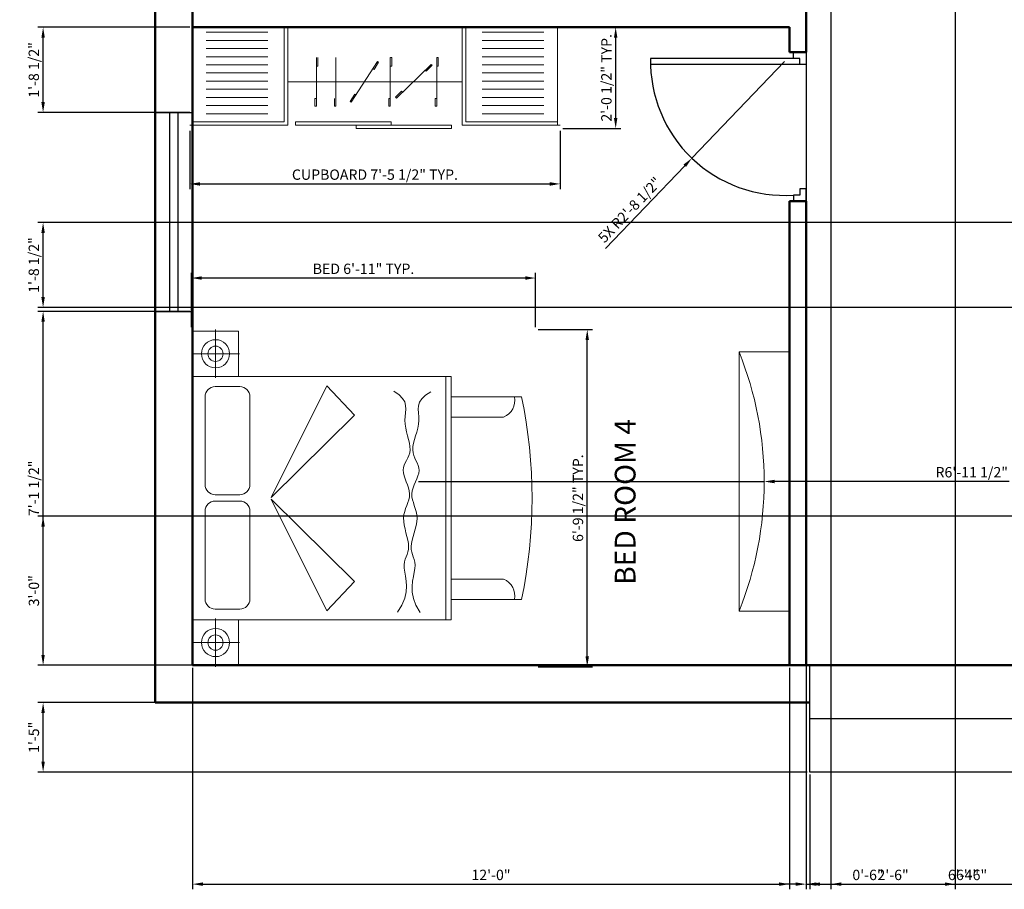
# Model space of a CAD drawing. Units: inches. Extents: x 1905 to 2315, y 3232 to 3824.
# Tile 1 of 8: x 1905 to 2143, y 3232 to 3442. Entities that reach past the tile are written whole.
import ezdxf

# ---------------------------------------------------------------- set-up
doc = ezdxf.new("R2010")
doc.units = ezdxf.units.IN
for name, color, linetype, lineweight in [('A-ANNO-DIMS', 2, 'Continuous', 18), ('A-AREA-IDEN', 7, 'Continuous', 25), ('A-FLOR-CABT', 8, 'Continuous', 18), ('A-FLOR-STRS', 7, 'Continuous', 25), ('A-FURN', 8, 'Continuous', 18), ('door', 1, 'Continuous', 25), ('TV', 221, 'Continuous', 18), ('wall', 2, 'Continuous', 50), ('WINDOW', 60, 'Continuous', 25)]:
    doc.layers.add(name, color=color, linetype=linetype, lineweight=lineweight)
doc.styles.get("Standard").update_dxf_attribs({"font": 'arial.ttf'})
doc.dimstyles.new('ISO-25', dxfattribs={"dimtxt": 2.5, "dimasz": 2.5, "dimexe": 1.25, "dimexo": 0.625, "dimtad": 1, "dimdec": 1, "dimlunit": 3, "dimtxsty": 'Standard', "dimcen": 2.5, "dimadec": 0, "dimazin": 0, "dimtfac": 1, "dimtdec": 1, "dimtmove": 0, "dimatfit": 3, "dimfxl": 1, "dimarcsym": 0})

# ---------------------------------------------------------------- blocks, each defined once
blk = doc.blocks.new('A$C4F543DC7')
for p, q in [((0.0134, 3.35, -0.1688), (3.3134, 3.35, -0.1688)), ((0.4634, 3.35, -0.1688), (0.0134, 3.35, -0.1688)), ((0.0134, 2.896, -0.1688), (0.0134, 3.35, -0.1688)), ((0.0134, 3.35, -0.1688), (0.0134, 2.896, -0.1688)), ((0.2381, 3.1233, -0.4388), (0.2381, 3.3614, -0.4388)), ((0.4634, 3.35, -0.1688), (0.4634, 0.8, -0.1688)), ((2.8634, 3.35, -0.1688), (0.4634, 3.35, -0.1688)), ((0.4634, 2.896, -0.1688), (0.4634, 3.35, -0.1688)), ((2.8634, 0.8, -0.1688), (2.8634, 3.35, -0.1688)), ((2.8634, 3.35, -0.1688), (3.3134, 3.35, -0.1688)), ((2.8634, 2.896, -0.1688), (2.8634, 3.35, -0.1688)), ((3.0888, 3.1233, -0.4388), (3.0888, 3.3614, -0.4388)), ((3.3134, 3.35, -0.1688), (3.3134, 2.896, -0.1688)), ((3.3134, 3.35, -0.1688), (3.3134, 2.896, -0.1688)), ((1.5354, 3.226, -0.1688), (0.6684, 3.226, -0.1688)), ((2.6644, 3.226, -0.1688), (1.7974, 3.226, -0.1688)), ((0.2381, 3.1233, -0.4388), (0, 3.1233, -0.4388)), ((0.2381, 3.1233, -0.4388), (0.4762, 3.1233, -0.4388)), ((0.2381, 3.1233, -0.4388), (0.2381, 2.8852, -0.4388)), ((0.5684, 3.126, -0.1688), (0.5684, 2.884, -0.1688)), ((1.6354, 2.884, -0.1688), (1.6354, 3.126, -0.1688)), ((1.6974, 3.126, -0.1688), (1.6974, 2.884, -0.1688)), ((2.7644, 2.884, -0.1688), (2.7644, 3.126, -0.1688)), ((3.0888, 3.1233, -0.4388), (2.8507, 3.1233, -0.4388)), ((3.0888, 3.1233, -0.4388), (3.0888, 2.8852, -0.4388)), ((3.0888, 3.1233, -0.4388), (3.3269, 3.1233, -0.4388)), ((0.4634, 2.896, -0.1688), (0.0134, 2.896, -0.1688)), ((0.0134, 2.896, -0.1688), (0.4634, 2.896, -0.1688)), ((0.4634, 0.8, -0.1688), (0.4634, 2.896, -0.1688)), ((2.8634, 2.896, -0.1688), (2.8634, 0.8, -0.1688)), ((3.3134, 2.896, -0.1688), (2.8634, 2.896, -0.1688)), ((3.3134, 2.896, -0.1688), (2.8634, 2.896, -0.1688)), ((0.6684, 2.784, -0.1688), (1.5354, 2.784, -0.1688)), ((1.7974, 2.784, -0.1688), (2.6644, 2.784, -0.1688)), ((1.6534, 2.573, -0.1688), (0.5504, 2.025, -0.1688)), ((0.8414, 1.752, -0.1688), (1.6534, 2.573, -0.1688)), ((2.4814, 1.752, -0.1688), (1.6694, 2.573, -0.1688)), ((1.6694, 2.573, -0.1688), (2.7724, 2.025, -0.1688)), ((0.5504, 2.025, -0.1688), (0.8414, 1.752, -0.1688)), ((2.7724, 2.025, -0.1688), (2.4814, 1.752, -0.1688)), ((2.683, 1.312, -0.1688), (2.7182, 1.3641, -0.1688)), ((0.5369, 1.3267, -0.1688), (0.6088, 1.2835, -0.1688)), ((0.6088, 1.2835, -0.1688), (0.6756, 1.2566, -0.1688)), ((1.3963, 1.2612, -0.1688), (1.4328, 1.2664, -0.1688)), ((1.4328, 1.2664, -0.1688), (1.4679, 1.2677, -0.1688)), ((1.4679, 1.2677, -0.1688), (1.501, 1.2643, -0.1688)), ((1.501, 1.2643, -0.1688), (1.5324, 1.257, -0.1688)), ((1.8557, 1.2531, -0.1688), (1.8849, 1.263, -0.1688)), ((1.8849, 1.263, -0.1688), (1.913, 1.2698, -0.1688)), ((1.913, 1.2698, -0.1688), (1.9397, 1.2722, -0.1688)), ((1.9397, 1.2722, -0.1688), (1.9649, 1.2692, -0.1688)), ((1.9649, 1.2692, -0.1688), (1.989, 1.2617, -0.1688)), ((2.6129, 1.257, -0.1688), (2.6479, 1.2774, -0.1688)), ((2.6479, 1.2774, -0.1688), (2.683, 1.312, -0.1688)), ((0.6067, 1.1458, -0.1688), (0.6743, 1.1706, -0.1688)), ((0.6743, 1.1706, -0.1688), (0.7364, 1.1825, -0.1688)), ((0.6756, 1.2566, -0.1688), (0.7373, 1.2428, -0.1688)), ((0.7364, 1.1825, -0.1688), (0.7931, 1.1846, -0.1688)), ((0.7373, 1.2428, -0.1688), (0.794, 1.239, -0.1688)), ((0.7931, 1.1846, -0.1688), (0.8447, 1.1799, -0.1688)), ((0.794, 1.239, -0.1688), (0.8457, 1.242, -0.1688)), ((0.8447, 1.1799, -0.1688), (0.8913, 1.1716, -0.1688)), ((0.8457, 1.242, -0.1688), (0.8925, 1.2489, -0.1688)), ((0.8913, 1.1716, -0.1688), (0.9331, 1.1628, -0.1688)), ((0.8925, 1.2489, -0.1688), (0.9345, 1.2564, -0.1688)), ((0.9345, 1.2564, -0.1688), (0.9718, 1.2615, -0.1688)), ((0.9718, 1.2615, -0.1688), (1.0044, 1.2617, -0.1688)), ((1.0044, 1.2617, -0.1688), (1.0334, 1.2578, -0.1688)), ((1.0334, 1.2578, -0.1688), (1.0597, 1.2509, -0.1688)), ((1.0583, 1.1642, -0.1688), (1.0831, 1.172, -0.1688)), ((1.0597, 1.2509, -0.1688), (1.0842, 1.2424, -0.1688)), ((1.0831, 1.172, -0.1688), (1.1072, 1.18, -0.1688)), ((1.0842, 1.2424, -0.1688), (1.1081, 1.2336, -0.1688)), ((1.1072, 1.18, -0.1688), (1.1316, 1.1872, -0.1688)), ((1.1081, 1.2336, -0.1688), (1.1322, 1.2257, -0.1688)), ((1.1316, 1.1872, -0.1688), (1.1573, 1.192, -0.1688)), ((1.1322, 1.2257, -0.1688), (1.1577, 1.2201, -0.1688)), ((1.1573, 1.192, -0.1688), (1.1851, 1.1932, -0.1688)), ((1.1577, 1.2201, -0.1688), (1.1855, 1.218, -0.1688)), ((1.1851, 1.1932, -0.1688), (1.2158, 1.1898, -0.1688)), ((1.1855, 1.218, -0.1688), (1.2163, 1.2204, -0.1688)), ((1.2158, 1.1898, -0.1688), (1.2491, 1.1828, -0.1688)), ((1.2163, 1.2204, -0.1688), (1.2498, 1.2264, -0.1688)), ((1.2491, 1.1828, -0.1688), (1.2842, 1.1734, -0.1688)), ((1.2498, 1.2264, -0.1688), (1.2852, 1.2347, -0.1688)), ((1.2842, 1.1734, -0.1688), (1.3206, 1.1629, -0.1688)), ((1.2852, 1.2347, -0.1688), (1.3218, 1.2441, -0.1688)), ((1.3218, 1.2441, -0.1688), (1.3591, 1.2533, -0.1688)), ((1.3591, 1.2533, -0.1688), (1.3963, 1.2612, -0.1688)), ((1.5324, 1.257, -0.1688), (1.5624, 1.2473, -0.1688)), ((1.5624, 1.2473, -0.1688), (1.5915, 1.2365, -0.1688)), ((1.5903, 1.1619, -0.1688), (1.6191, 1.1716, -0.1688)), ((1.5915, 1.2365, -0.1688), (1.6199, 1.2259, -0.1688)), ((1.6191, 1.1716, -0.1688), (1.6475, 1.1797, -0.1688)), ((1.6199, 1.2259, -0.1688), (1.6481, 1.2169, -0.1688)), ((1.6475, 1.1797, -0.1688), (1.676, 1.1849, -0.1688)), ((1.6481, 1.2169, -0.1688), (1.6765, 1.2108, -0.1688)), ((1.676, 1.1849, -0.1688), (1.7049, 1.1858, -0.1688)), ((1.6765, 1.2108, -0.1688), (1.7053, 1.209, -0.1688)), ((1.7049, 1.1858, -0.1688), (1.7344, 1.1816, -0.1688)), ((1.7053, 1.209, -0.1688), (1.7349, 1.2124, -0.1688)), ((1.7344, 1.1816, -0.1688), (1.7643, 1.1731, -0.1688)), ((1.7349, 1.2124, -0.1688), (1.7651, 1.2199, -0.1688)), ((1.7643, 1.1731, -0.1688), (1.7944, 1.1619, -0.1688)), ((1.7651, 1.2199, -0.1688), (1.7955, 1.2301, -0.1688)), ((1.7955, 1.2301, -0.1688), (1.8258, 1.2417, -0.1688)), ((1.8258, 1.2417, -0.1688), (1.8557, 1.2531, -0.1688)), ((1.989, 1.2617, -0.1688), (2.0124, 1.2512, -0.1688)), ((2.0124, 1.2512, -0.1688), (2.0359, 1.2391, -0.1688)), ((2.0359, 1.2391, -0.1688), (2.0599, 1.2269, -0.1688)), ((2.0588, 1.1568, -0.1688), (2.0842, 1.167, -0.1688)), ((2.0599, 1.2269, -0.1688), (2.0849, 1.216, -0.1688)), ((2.0842, 1.167, -0.1688), (2.1112, 1.1743, -0.1688)), ((2.0849, 1.216, -0.1688), (2.1117, 1.2077, -0.1688)), ((2.1112, 1.1743, -0.1688), (2.1403, 1.1775, -0.1688)), ((2.1117, 1.2077, -0.1688), (2.1407, 1.2037, -0.1688)), ((2.1403, 1.1775, -0.1688), (2.1718, 1.1755, -0.1688)), ((2.1407, 1.2037, -0.1688), (2.1723, 1.2047, -0.1688)), ((2.1718, 1.1755, -0.1688), (2.2056, 1.1691, -0.1688)), ((2.1723, 1.2047, -0.1688), (2.2062, 1.21, -0.1688)), ((2.2056, 1.1691, -0.1688), (2.2411, 1.1598, -0.1688)), ((2.2062, 1.21, -0.1688), (2.242, 1.2182, -0.1688)), ((2.242, 1.2182, -0.1688), (2.2791, 1.2279, -0.1688)), ((2.2791, 1.2279, -0.1688), (2.3173, 1.2378, -0.1688)), ((2.3173, 1.2378, -0.1688), (2.3558, 1.2465, -0.1688)), ((2.3558, 1.2465, -0.1688), (2.3944, 1.2527, -0.1688)), ((2.3944, 1.2527, -0.1688), (2.4325, 1.255, -0.1688)), ((2.4325, 1.255, -0.1688), (2.4698, 1.2529, -0.1688)), ((2.4698, 1.2529, -0.1688), (2.5064, 1.2488, -0.1688)), ((2.5064, 1.2488, -0.1688), (2.5423, 1.2459, -0.1688)), ((2.5423, 1.2459, -0.1688), (2.5777, 1.2476, -0.1688)), ((2.5777, 1.2476, -0.1688), (2.6129, 1.257, -0.1688)), ((0.5334, 1.105, -0.1688), (0.6067, 1.1458, -0.1688)), ((0.9331, 1.1628, -0.1688), (0.9701, 1.1565, -0.1688)), ((0.9701, 1.1565, -0.1688), (1.0027, 1.1552, -0.1688)), ((1.0027, 1.1552, -0.1688), (1.0318, 1.1582, -0.1688)), ((1.0318, 1.1582, -0.1688), (1.0583, 1.1642, -0.1688)), ((1.3206, 1.1629, -0.1688), (1.3575, 1.1524, -0.1688)), ((1.3575, 1.1524, -0.1688), (1.3945, 1.1434, -0.1688)), ((1.3945, 1.1434, -0.1688), (1.4308, 1.1371, -0.1688)), ((1.4308, 1.1371, -0.1688), (1.4658, 1.1347, -0.1688)), ((1.4658, 1.1347, -0.1688), (1.499, 1.137, -0.1688)), ((1.499, 1.137, -0.1688), (1.5306, 1.1433, -0.1688)), ((1.5306, 1.1433, -0.1688), (1.5609, 1.152, -0.1688)), ((1.5609, 1.152, -0.1688), (1.5903, 1.1619, -0.1688)), ((1.7944, 1.1619, -0.1688), (1.8244, 1.1494, -0.1688)), ((1.8244, 1.1494, -0.1688), (1.8539, 1.137, -0.1688)), ((1.8539, 1.137, -0.1688), (1.8827, 1.1263, -0.1688)), ((1.8827, 1.1263, -0.1688), (1.9106, 1.1186, -0.1688)), ((1.9106, 1.1186, -0.1688), (1.9373, 1.1153, -0.1688)), ((1.9373, 1.1153, -0.1688), (1.9625, 1.1176, -0.1688)), ((1.9625, 1.1176, -0.1688), (1.9868, 1.1243, -0.1688)), ((1.9868, 1.1243, -0.1688), (2.0106, 1.134, -0.1688)), ((2.0106, 1.134, -0.1688), (2.0344, 1.1454, -0.1688)), ((2.0344, 1.1454, -0.1688), (2.0588, 1.1568, -0.1688)), ((2.2411, 1.1598, -0.1688), (2.2779, 1.1489, -0.1688)), ((2.2779, 1.1489, -0.1688), (2.3157, 1.1379, -0.1688)), ((2.3157, 1.1379, -0.1688), (2.354, 1.1279, -0.1688)), ((2.354, 1.1279, -0.1688), (2.3923, 1.1205, -0.1688)), ((2.3923, 1.1205, -0.1688), (2.4304, 1.117, -0.1688)), ((2.4304, 1.117, -0.1688), (2.4677, 1.118, -0.1688)), ((2.4677, 1.118, -0.1688), (2.5043, 1.1209, -0.1688)), ((2.5043, 1.1209, -0.1688), (2.5403, 1.1226, -0.1688)), ((2.5403, 1.1226, -0.1688), (2.5757, 1.1199, -0.1688)), ((2.5757, 1.1199, -0.1688), (2.6106, 1.1094, -0.1688)), ((2.6106, 1.1094, -0.1688), (2.645, 1.0879, -0.1688)), ((2.645, 1.0879, -0.1688), (2.6789, 1.0522, -0.1688)), ((2.6789, 1.0522, -0.1688), (2.7124, 0.999, -0.1688)), ((0.4634, 0.85, -0.1688), (2.8634, 0.85, -0.1688)), ((0.4634, 0.8, -0.1688), (2.8634, 0.8, -0.1688)), ((0.6634, 0.8, -0.1688), (0.4634, 0.8, -0.1688)), ((0.6634, 0.8, -0.1688), (2.6634, 0.8, -0.1688)), ((0.6634, 0.104, -0.1688), (0.6634, 0.8, -0.1688)), ((0.6634, 0.104, -0.1688), (0.6634, 0.8, -0.1688)), ((0.8634, 0.281, -0.1688), (0.8634, 0.8, -0.1688)), ((2.4634, 0.8, -0.1688), (2.4634, 0.281, -0.1688)), ((2.8634, 0.8, -0.1688), (2.6634, 0.8, -0.1688)), ((2.6634, 0.8, -0.1688), (2.6634, 0.104, -0.1688)), ((2.6634, 0.8, -0.1688), (2.6634, 0.104, -0.1688))]:
    blk.add_line(p, q)
for centre, radius in [((0.2381, 3.1233, -0.4388), 0.139), ((3.0888, 3.1233, -0.4388), 0.139), ((0.2381, 3.1233, -0.4388), 0.075), ((3.0888, 3.1233, -0.4388), 0.075)]:
    blk.add_circle(centre, radius)
for centre, radius, start, end in [((0.6684, 3.126, -0.1688), 0.1, 90, 180), ((1.5354, 3.126, -0.1688), 0.1, 0, 90), ((1.7974, 3.126, -0.1688), 0.1, 90, 180), ((2.6644, 3.126, -0.1688), 0.1, 0, 90), ((0.6684, 2.884, -0.1688), 0.1, 180, 270), ((1.5354, 2.884, -0.1688), 0.1, 270, 0), ((1.7974, 2.884, -0.1688), 0.1, 180, 270), ((2.6644, 2.884, -0.1688), 0.1, 270, 0), ((0.6994, 0.3472, -0.1688), 0.1769, 258.2616, 338.03196), ((2.6275, 0.3472, -0.1688), 0.1769, 201.96804, 281.7384), ((1.6634, 4.8597, -0.1688), 4.8597, 258.12517, 281.87483), ((1.6634, 4.8597, -0.1688), 4.8597, 258.12517, 281.87483)]:
    blk.add_arc(centre, radius, start, end)
blk = doc.blocks.new('CUPBOARD-DOUBLE-BAY')
at = {"ltscale": 0.05}
for p, q in [((88.68, 24.41), (0.66, 24.41)), ((0.66, 0.79), (0.66, 24.41)), ((88.68, 0.79), (88.68, 24.41)), ((48.39, 17.11), (48.73, 17.11)), ((59.57, 17.11), (59.9, 17.11)), ((30.53, 15.05), (30.86, 15.05)), ((44.17, 14.43), (44.45, 14.25)), ((45.28, 16.16), (45.56, 15.98)), ((48.39, 15.05), (48.73, 15.05)), ((58.24, 15.47), (58.47, 15.23)), ((59.57, 15.05), (59.9, 15.05)), ((56.76, 14.03), (56.99, 13.79)), ((30.53, 7.22), (30.19, 7.22)), ((40.06, 8.06), (39.78, 8.24)), ((48.35, 7.22), (48.02, 7.22)), ((49.85, 7.29), (49.61, 7.53)), ((51.32, 8.73), (51.09, 8.97)), ((59.57, 7.22), (59.23, 7.22)), ((30.53, 5.41), (30.19, 5.41)), ((35.23, 5.41), (34.9, 5.41)), ((38.95, 6.33), (38.67, 6.51)), ((48.35, 5.41), (48.02, 5.41)), ((59.57, 5.41), (59.23, 5.41))]:
    blk.add_line(p, q, dxfattribs=at)
for p, q in [((22.77, 1.58), (22.77, 24.41)), ((23.62, 0.79), (23.62, 24.41)), ((65.72, 0.79), (65.72, 24.41)), ((66.57, 1.58), (66.57, 24.41)), ((18.83, 23.23), (3.94, 23.23)), ((70.51, 23.23), (85.4, 23.23)), ((18.83, 21.26), (3.94, 21.26)), ((18.83, 19.29), (3.94, 19.29)), ((70.51, 21.26), (85.4, 21.26)), ((70.51, 19.29), (85.4, 19.29)), ((18.83, 17.32), (3.94, 17.32)), ((30.53, 5.41), (30.53, 17.11)), ((30.86, 15.05), (30.86, 17.11)), ((35.23, 5.41), (35.23, 17.11)), ((48.35, 5.41), (48.35, 17.11)), ((48.73, 15.05), (48.73, 17.11)), ((59.57, 5.41), (59.57, 17.11)), ((59.9, 15.05), (59.9, 17.11)), ((70.51, 17.32), (85.4, 17.32)), ((18.83, 15.35), (3.94, 15.35)), ((38.95, 6.33), (45.28, 16.16)), ((44.45, 14.25), (45.56, 15.98)), ((49.85, 7.29), (58.22, 15.46)), ((56.99, 13.79), (58.47, 15.23)), ((70.51, 15.35), (85.4, 15.35)), ((18.83, 13.39), (3.94, 13.39)), ((70.51, 13.39), (85.4, 13.39)), ((18.83, 11.42), (3.94, 11.42)), ((65.6, 11.21), (23.75, 11.21)), ((70.51, 11.42), (85.4, 11.42)), ((18.83, 9.45), (3.94, 9.45)), ((18.83, 7.48), (3.94, 7.48)), ((30.19, 7.22), (30.19, 5.41)), ((34.9, 7.22), (34.9, 5.41)), ((38.67, 6.51), (39.78, 8.24)), ((48.02, 7.22), (48.02, 5.41)), ((49.61, 7.53), (51.09, 8.97)), ((59.23, 7.22), (59.23, 5.41)), ((70.51, 9.45), (85.4, 9.45)), ((70.51, 7.48), (85.4, 7.48)), ((18.83, 5.51), (3.94, 5.51)), ((70.51, 5.51), (85.4, 5.51)), ((18.83, 3.54), (3.94, 3.54)), ((70.51, 3.54), (85.4, 3.54)), ((23.62, 0.79), (0, 0.79)), ((22.77, 1.58), (0.66, 1.58)), ((25.54, 1.58), (25.54, 0.79)), ((48.56, 1.58), (25.54, 1.58)), ((25.54, 0.79), (48.56, 0.79)), ((40.11, 0), (40.11, 0.79)), ((40.11, 0.79), (63.12, 0.79)), ((63.12, 0), (40.11, 0)), ((48.56, 0.79), (48.56, 1.58)), ((63.12, 0.79), (63.12, 0)), ((65.72, 0.79), (89.34, 0.79)), ((66.57, 1.58), (88.68, 1.58))]:
    blk.add_line(p, q)
blk = doc.blocks.new('DOOR-SWING-36IN')
for p, q in [((34.51, 36), (37.51, 36)), ((34.51, 34.5), (34.51, 36)), ((37.51, 36), (37.51, 33)), ((36.01, 34.5), (0.01, 34.5)), ((36.01, 34.5), (34.51, 34.5)), ((36.01, 33), (36.01, 34.5)), ((36.01, 33), (0.01, 33)), ((37.51, 33), (36.01, 33)), ((37.51, 3), (36.01, 3)), ((36.01, 3), (36.01, 1.5)), ((37.51, 0), (37.51, 3)), ((36.01, 1.5), (34.51, 1.5)), ((34.51, 1.5), (34.51, 0)), ((34.51, 0), (37.51, 0))]:
    blk.add_line(p, q)
blk.add_arc((32.32, 33.75), 32.32, 178.6705, 273.8756)
blk = doc.blocks.new('WIN-48IN')
for p, q in [((0, 9), (0, 0)), ((0, 9), (48, 9)), ((48, 9), (48, 0)), ((0, 5.5), (48, 5.5)), ((0, 3.5), (48, 3.5)), ((0, 0), (48, 0))]:
    blk.add_line(p, q)
blk = doc.blocks.new('*D27')
at = {"layer": 'A-ANNO-DIMS', "color": 0, "lineweight": -2, "transparency": 16777216}
for p, q in [((1946.73, 3367.88), (1946.73, 3380.96)), ((2029.77, 3367.88), (2029.77, 3380.96)), ((2027.27, 3379.71), (1949.23, 3379.71))]:
    blk.add_line(p, q, dxfattribs=at)
at = {"layer": 'A-ANNO-DIMS', "color": 0, "transparency": 16777216}
for points in [[(1949.23, 3380.13), (1949.23, 3379.29), (1946.73, 3379.71)], [(2027.27, 3380.13), (2027.27, 3379.29), (2029.77, 3379.71)]]:
    blk.add_solid(points, dxfattribs=at)
at = {"layer": 'Defpoints', "color": 0, "transparency": 16777216}
for p in [(1946.73, 3379.71), (1946.73, 3367.25), (2029.77, 3367.25)]:
    blk.add_point(p, dxfattribs=at)
at = {"layer": 'A-ANNO-DIMS', "color": 0, "transparency": 16777216, "insert": (1988.25, 3381.61), "char_height": 2.5, "attachment_point": 5}
blk.add_mtext('BED 6\'-11" TYP.', dxfattribs=at)
blk = doc.blocks.new('*D28')
at = {"layer": 'A-ANNO-DIMS', "color": 0, "lineweight": -2, "transparency": 16777216}
for p, q in [((2030.4, 3367.25), (2043.48, 3367.25)), ((2042.23, 3288.4), (2042.23, 3364.75)), ((2030.4, 3285.9), (2043.48, 3285.9))]:
    blk.add_line(p, q, dxfattribs=at)
at = {"layer": 'A-ANNO-DIMS', "color": 0, "transparency": 16777216}
for points in [[(2041.81, 3364.75), (2042.64, 3364.75), (2042.23, 3367.25)], [(2041.81, 3288.4), (2042.64, 3288.4), (2042.23, 3285.9)]]:
    blk.add_solid(points, dxfattribs=at)
at = {"layer": 'Defpoints', "color": 0, "transparency": 16777216}
for p in [(2029.77, 3367.25), (2042.23, 3367.25), (2029.77, 3285.9)]:
    blk.add_point(p, dxfattribs=at)
at = {"layer": 'A-ANNO-DIMS', "color": 0, "transparency": 16777216, "insert": (2040.31, 3326.58), "char_height": 2.5, "attachment_point": 5, "rotation": 90}
blk.add_mtext('6\'-9 1/2" TYP.', dxfattribs=at)
blk = doc.blocks.new('*D29')
at = {"layer": 'A-ANNO-DIMS', "color": 0, "lineweight": -2, "transparency": 16777216}
for p, q in [((1946.34, 3415.2), (1946.34, 3401.17)), ((2035.69, 3415.2), (2035.69, 3401.17)), ((1948.84, 3402.42), (2033.19, 3402.42))]:
    blk.add_line(p, q, dxfattribs=at)
at = {"layer": 'A-ANNO-DIMS', "color": 0, "transparency": 16777216}
for points in [[(1948.84, 3402.84), (1948.84, 3402), (1946.34, 3402.42)], [(2033.19, 3402.84), (2033.19, 3402), (2035.69, 3402.42)]]:
    blk.add_solid(points, dxfattribs=at)
at = {"layer": 'Defpoints', "color": 0, "transparency": 16777216}
for p in [(1946.34, 3415.82), (2035.69, 3415.82), (2035.69, 3402.42)]:
    blk.add_point(p, dxfattribs=at)
at = {"layer": 'A-ANNO-DIMS', "color": 0, "transparency": 16777216, "insert": (1991.01, 3404.34), "char_height": 2.5, "attachment_point": 5}
blk.add_mtext('CUPBOARD 7\'-5 1/2" TYP.', dxfattribs=at)
blk = doc.blocks.new('*D30')
at = {"layer": 'A-ANNO-DIMS', "color": 0, "lineweight": -2, "transparency": 16777216}
for p, q in [((2036.31, 3440.23), (2050.34, 3440.23)), ((2049.09, 3418.32), (2049.09, 3437.73)), ((2036.31, 3415.82), (2050.34, 3415.82))]:
    blk.add_line(p, q, dxfattribs=at)
at = {"layer": 'A-ANNO-DIMS', "color": 0, "transparency": 16777216}
for points in [[(2048.67, 3437.73), (2049.5, 3437.73), (2049.09, 3440.23)], [(2048.67, 3418.32), (2049.5, 3418.32), (2049.09, 3415.82)]]:
    blk.add_solid(points, dxfattribs=at)
at = {"layer": 'Defpoints', "color": 0, "transparency": 16777216}
for p in [(2035.69, 3440.23), (2049.09, 3440.23), (2035.69, 3415.82)]:
    blk.add_point(p, dxfattribs=at)
at = {"layer": 'A-ANNO-DIMS', "color": 0, "transparency": 16777216, "insert": (2047.17, 3428.03), "char_height": 2.5, "attachment_point": 5, "rotation": 90}
blk.add_mtext('2\'-0 1/2" TYP.', dxfattribs=at)
blk = doc.blocks.new('*D41')
at = {"layer": 'A-ANNO-DIMS', "color": 0, "lineweight": -2, "transparency": 16777216}
for p, q in [((2095.01, 3663.61), (2095.01, 3232.16)), ((2171.01, 3663.61), (2171.01, 3232.16)), ((2097.51, 3233.41), (2168.51, 3233.41))]:
    blk.add_line(p, q, dxfattribs=at)
at = {"layer": 'A-ANNO-DIMS', "color": 0, "transparency": 16777216}
for points in [[(2097.51, 3233.83), (2097.51, 3233), (2095.01, 3233.41)], [(2168.51, 3233.83), (2168.51, 3233), (2171.01, 3233.41)]]:
    blk.add_solid(points, dxfattribs=at)
at = {"layer": 'Defpoints', "color": 0, "transparency": 16777216}
for p in [(2095.01, 3664.23), (2171.01, 3664.23), (2171.01, 3233.41)]:
    blk.add_point(p, dxfattribs=at)
at = {"layer": 'A-ANNO-DIMS', "color": 0, "transparency": 16777216, "insert": (2133.01, 3235.31), "char_height": 2.5, "attachment_point": 5}
blk.add_mtext('6\'-4"', dxfattribs=at)
blk = doc.blocks.new('*D44')
at = {"layer": 'A-ANNO-DIMS', "color": 0, "lineweight": -2, "transparency": 16777216}
for p, q in [((1946.38, 3371.66), (1909.7, 3371.66)), ((1910.95, 3288.73), (1910.95, 3369.16)), ((1946.38, 3286.23), (1909.7, 3286.23))]:
    blk.add_line(p, q, dxfattribs=at)
at = {"layer": 'A-ANNO-DIMS', "color": 0, "transparency": 16777216}
for points in [[(1910.53, 3369.16), (1911.36, 3369.16), (1910.95, 3371.66)], [(1910.53, 3288.73), (1911.36, 3288.73), (1910.95, 3286.23)]]:
    blk.add_solid(points, dxfattribs=at)
at = {"layer": 'Defpoints', "color": 0, "transparency": 16777216}
for p in [(1910.95, 3371.66), (1947.01, 3371.66), (1947.01, 3286.23)]:
    blk.add_point(p, dxfattribs=at)
at = {"layer": 'A-ANNO-DIMS', "color": 0, "transparency": 16777216, "insert": (1909.03, 3328.94), "char_height": 2.5, "attachment_point": 5, "rotation": 90}
blk.add_mtext('7\'-1 1/2"', dxfattribs=at)
blk = doc.blocks.new('*D45')
at = {"layer": 'A-ANNO-DIMS', "color": 0, "lineweight": -2, "transparency": 16777216}
for p, q in [((1946.38, 3440.23), (1909.7, 3440.23)), ((1910.95, 3422.16), (1910.95, 3437.73)), ((1946.38, 3419.66), (1909.7, 3419.66))]:
    blk.add_line(p, q, dxfattribs=at)
at = {"layer": 'A-ANNO-DIMS', "color": 0, "transparency": 16777216}
for points in [[(1910.53, 3437.73), (1911.36, 3437.73), (1910.95, 3440.23)], [(1910.53, 3422.16), (1911.36, 3422.16), (1910.95, 3419.66)]]:
    blk.add_solid(points, dxfattribs=at)
at = {"layer": 'Defpoints', "color": 0, "transparency": 16777216}
for p in [(1910.95, 3440.23), (1947.01, 3440.23), (1947.01, 3419.66)]:
    blk.add_point(p, dxfattribs=at)
at = {"layer": 'A-ANNO-DIMS', "color": 0, "transparency": 16777216, "insert": (1909.03, 3429.94), "char_height": 2.5, "attachment_point": 5, "rotation": 90}
blk.add_mtext('1\'-8 1/2"', dxfattribs=at)
blk = doc.blocks.new('*D56')
at = {"layer": 'A-ANNO-DIMS', "color": 0, "lineweight": -2, "transparency": 16777216}
for p, q in [((1947.01, 3285.61), (1947.01, 3232.16)), ((2091.01, 3285.61), (2091.01, 3232.16)), ((1949.51, 3233.41), (2088.51, 3233.41))]:
    blk.add_line(p, q, dxfattribs=at)
at = {"layer": 'A-ANNO-DIMS', "color": 0, "transparency": 16777216}
for points in [[(1949.51, 3233.83), (1949.51, 3233), (1947.01, 3233.41)], [(2088.51, 3233.83), (2088.51, 3233), (2091.01, 3233.41)]]:
    blk.add_solid(points, dxfattribs=at)
at = {"layer": 'Defpoints', "color": 0, "transparency": 16777216}
for p in [(1947.01, 3286.23), (2091.01, 3286.23), (2091.01, 3233.41)]:
    blk.add_point(p, dxfattribs=at)
at = {"layer": 'A-ANNO-DIMS', "color": 0, "transparency": 16777216, "insert": (2019.01, 3235.31), "char_height": 2.5, "attachment_point": 5}
blk.add_mtext('12\'-0"', dxfattribs=at)
blk = doc.blocks.new('*D57')
at = {"layer": 'A-ANNO-DIMS', "color": 0, "lineweight": -2, "transparency": 16777216}
for p, q in [((2095.91, 3259.85), (2095.91, 3232.16)), ((2173.99, 3259.85), (2173.99, 3232.16)), ((2098.41, 3233.41), (2171.49, 3233.41))]:
    blk.add_line(p, q, dxfattribs=at)
at = {"layer": 'A-ANNO-DIMS', "color": 0, "transparency": 16777216}
for points in [[(2098.41, 3233.83), (2098.41, 3233), (2095.91, 3233.41)], [(2171.49, 3233.83), (2171.49, 3233), (2173.99, 3233.41)]]:
    blk.add_solid(points, dxfattribs=at)
at = {"layer": 'Defpoints', "color": 0, "transparency": 16777216}
for p in [(2095.91, 3260.47), (2173.99, 3260.47), (2173.99, 3233.41)]:
    blk.add_point(p, dxfattribs=at)
at = {"layer": 'A-ANNO-DIMS', "color": 0, "transparency": 16777216, "insert": (2134.95, 3235.31), "char_height": 2.5, "attachment_point": 5}
blk.add_mtext('6\'-6"', dxfattribs=at)
blk = doc.blocks.new('*D59')
at = {"layer": 'A-ANNO-DIMS', "color": 0, "lineweight": -2, "transparency": 16777216}
for p, q in [((2095.29, 3277.23), (1909.7, 3277.23)), ((1910.95, 3262.97), (1910.95, 3274.73)), ((2095.29, 3260.47), (1909.7, 3260.47))]:
    blk.add_line(p, q, dxfattribs=at)
at = {"layer": 'A-ANNO-DIMS', "color": 0, "transparency": 16777216}
for points in [[(1910.53, 3274.73), (1911.36, 3274.73), (1910.95, 3277.23)], [(1910.53, 3262.97), (1911.36, 3262.97), (1910.95, 3260.47)]]:
    blk.add_solid(points, dxfattribs=at)
at = {"layer": 'Defpoints', "color": 0, "transparency": 16777216}
for p in [(1910.95, 3277.23), (2095.91, 3277.23), (2095.91, 3260.47)]:
    blk.add_point(p, dxfattribs=at)
at = {"layer": 'A-ANNO-DIMS', "color": 0, "transparency": 16777216, "insert": (1909.05, 3268.85), "char_height": 2.5, "attachment_point": 5, "rotation": 90}
blk.add_mtext('1\'-5"', dxfattribs=at)
blk = doc.blocks.new('*D61')
at = {"layer": 'A-ANNO-DIMS', "color": 0, "lineweight": -2, "transparency": 16777216}
for p, q in [((2176.38, 3322.23), (1909.7, 3322.23)), ((1910.95, 3288.73), (1910.95, 3319.73)), ((2176.38, 3286.23), (1909.7, 3286.23))]:
    blk.add_line(p, q, dxfattribs=at)
at = {"layer": 'A-ANNO-DIMS', "color": 0, "transparency": 16777216}
for points in [[(1910.53, 3319.73), (1911.36, 3319.73), (1910.95, 3322.23)], [(1910.53, 3288.73), (1911.36, 3288.73), (1910.95, 3286.23)]]:
    blk.add_solid(points, dxfattribs=at)
at = {"layer": 'Defpoints', "color": 0, "transparency": 16777216}
for p in [(1910.95, 3322.23), (2177.01, 3322.23), (2177.01, 3286.23)]:
    blk.add_point(p, dxfattribs=at)
at = {"layer": 'A-ANNO-DIMS', "color": 0, "transparency": 16777216, "insert": (1909.05, 3304.23), "char_height": 2.5, "attachment_point": 5, "rotation": 90}
blk.add_mtext('3\'-0"', dxfattribs=at)
blk = doc.blocks.new('*D64')
at = {"layer": 'A-ANNO-DIMS', "color": 0, "lineweight": -2, "transparency": 16777216}
for p, q in [((2101.01, 3659.61), (2101.01, 3232.16)), ((2131.01, 3659.61), (2131.01, 3232.16)), ((2103.51, 3233.41), (2128.51, 3233.41))]:
    blk.add_line(p, q, dxfattribs=at)
at = {"layer": 'A-ANNO-DIMS', "color": 0, "transparency": 16777216}
for points in [[(2103.51, 3233.83), (2103.51, 3233), (2101.01, 3233.41)], [(2128.51, 3233.83), (2128.51, 3233), (2131.01, 3233.41)]]:
    blk.add_solid(points, dxfattribs=at)
at = {"layer": 'Defpoints', "color": 0, "transparency": 16777216}
for p in [(2101.01, 3660.23), (2131.01, 3660.23), (2131.01, 3233.41)]:
    blk.add_point(p, dxfattribs=at)
at = {"layer": 'A-ANNO-DIMS', "color": 0, "transparency": 16777216, "insert": (2116.01, 3235.31), "char_height": 2.5, "attachment_point": 5}
blk.add_mtext('2\'-6"', dxfattribs=at)
blk = doc.blocks.new('*D65')
at = {"layer": 'A-ANNO-DIMS', "color": 0, "lineweight": -2, "transparency": 16777216}
for p, q in [((2095.01, 3659.61), (2095.01, 3232.16)), ((2101.01, 3659.61), (2101.01, 3232.16)), ((2092.51, 3233.41), (2090.01, 3233.41)), ((2095.01, 3233.41), (2101.01, 3233.41)), ((2103.51, 3233.41), (2113.9, 3233.41))]:
    blk.add_line(p, q, dxfattribs=at)
at = {"layer": 'A-ANNO-DIMS', "color": 0, "transparency": 16777216}
for points in [[(2092.51, 3233.83), (2092.51, 3233), (2095.01, 3233.41)], [(2103.51, 3233.83), (2103.51, 3233), (2101.01, 3233.41)]]:
    blk.add_solid(points, dxfattribs=at)
at = {"layer": 'Defpoints', "color": 0, "transparency": 16777216}
for p in [(2095.01, 3660.23), (2101.01, 3660.23), (2101.01, 3233.41)]:
    blk.add_point(p, dxfattribs=at)
at = {"layer": 'A-ANNO-DIMS', "color": 0, "transparency": 16777216, "insert": (2109.96, 3235.31), "char_height": 2.5, "attachment_point": 5}
blk.add_mtext('0\'-6"', dxfattribs=at)
blk = doc.blocks.new('*D67')
at = {"layer": 'A-ANNO-DIMS', "color": 0, "lineweight": -2, "transparency": 16777216}
for p, q in [((2174.38, 3393.11), (1909.7, 3393.11)), ((1910.95, 3375.1), (1910.95, 3390.61)), ((2174.38, 3372.6), (1909.7, 3372.6))]:
    blk.add_line(p, q, dxfattribs=at)
at = {"layer": 'A-ANNO-DIMS', "color": 0, "transparency": 16777216}
for points in [[(1910.53, 3390.61), (1911.36, 3390.61), (1910.95, 3393.11)], [(1910.53, 3375.1), (1911.36, 3375.1), (1910.95, 3372.6)]]:
    blk.add_solid(points, dxfattribs=at)
at = {"layer": 'Defpoints', "color": 0, "transparency": 16777216}
for p in [(1910.95, 3393.11), (2175.01, 3393.11), (2175.01, 3372.6)]:
    blk.add_point(p, dxfattribs=at)
at = {"layer": 'A-ANNO-DIMS', "color": 0, "transparency": 16777216, "insert": (1909.03, 3382.85), "char_height": 2.5, "attachment_point": 5, "rotation": 90}
blk.add_mtext('1\'-8 1/2"', dxfattribs=at)
blk = doc.blocks.new('*D74')
at = {"layer": 'A-ANNO-DIMS', "color": 0, "lineweight": -2, "transparency": 16777216}
for p, q in [((2089.82, 3431.98), (2067.48, 3408.62)), ((2046.65, 3386.84), (2065.75, 3406.82))]:
    blk.add_line(p, q, dxfattribs=at)
at = {"layer": 'A-ANNO-DIMS', "color": 0, "transparency": 16777216}
blk.add_solid([(2065.45, 3407.1), (2066.05, 3406.53), (2067.48, 3408.62)], dxfattribs=at)
at = {"layer": 'Defpoints', "color": 0, "transparency": 16777216}
for p in [(2089.82, 3431.98), (2067.48, 3408.62)]:
    blk.add_point(p, dxfattribs=at)
at = {"layer": 'A-ANNO-DIMS', "color": 0, "transparency": 16777216, "insert": (2052.69, 3395.93), "char_height": 2.5, "attachment_point": 5, "rotation": 46.2735}
blk.add_mtext('5X R2\'-8 1/2"', dxfattribs=at)
blk = doc.blocks.new('*D79')
at = {"layer": 'A-ANNO-DIMS', "color": 0, "lineweight": -2, "transparency": 16777216}
for p, q in [((2001.48, 3330.59), (2084.93, 3330.59)), ((2144.02, 3330.59), (2087.43, 3330.59))]:
    blk.add_line(p, q, dxfattribs=at)
at = {"layer": 'A-ANNO-DIMS', "color": 0, "transparency": 16777216}
blk.add_solid([(2087.43, 3331.01), (2087.43, 3330.17), (2084.93, 3330.59)], dxfattribs=at)
at = {"layer": 'Defpoints', "color": 0, "transparency": 16777216}
for p in [(2001.48, 3330.59), (2084.93, 3330.59)]:
    blk.add_point(p, dxfattribs=at)
at = {"layer": 'A-ANNO-DIMS', "color": 0, "transparency": 16777216, "insert": (2134.99, 3332.51), "char_height": 2.5, "attachment_point": 5, "rotation": 0.0001}
blk.add_mtext('R6\'-11 1/2"', dxfattribs=at)

msp = doc.modelspace()

# ---------------------------------------------------------------- linework, layer by layer
at = {"layer": 'A-FLOR-STRS'}
msp.add_line((2095.91, 3273.38), (2173.99, 3273.38), dxfattribs=at)
msp.add_lwpolyline([(2095.91, 3286.29), (2173.99, 3286.29), (2173.99, 3260.47), (2095.91, 3260.47)], close=True, dxfattribs=at)
at = {"layer": 'TV'}
msp.add_lwpolyline([(2091.01, 3361.86), (2078.85, 3361.86), (2078.85, 3299.32), (2091.01, 3299.32)], close=True, dxfattribs=at)
msp.add_arc((2001.48, 3330.59), 83.44, 337.9905, 22.0095, dxfattribs=at)
at = {"layer": 'wall'}
for p, q in [((1938.01, 3793.23), (1938.01, 3277.23)), ((1947.01, 3784.23), (1947.01, 3286.23)), ((2095.01, 3570.23), (2095.01, 3434.23)), ((2091.01, 3440.23), (1947.01, 3440.23)), ((2091.01, 3440.23), (2091.01, 3434.23)), ((2091.01, 3434.23), (2095.01, 3434.23)), ((2091.01, 3434.23), (2095.01, 3434.23)), ((2091.01, 3398.23), (2095.01, 3398.23)), ((2091.01, 3398.23), (2091.01, 3286.23)), ((2095.01, 3398.23), (2095.01, 3286.23)), ((1947.01, 3286.23), (2277.01, 3286.23)), ((1938.01, 3277.23), (2095.91, 3277.23))]:
    msp.add_line(p, q, dxfattribs=at)

# ---------------------------------------------------------------- block references
at = {"layer": 'A-FLOR-CABT'}
msp.add_blockref('CUPBOARD-DOUBLE-BAY', (1946.34, 3415.82), dxfattribs=at)
at = {"layer": 'A-FURN', "xscale": 24.45263891714, "yscale": 24.45263891714, "zscale": 24.45263891714, "rotation": 90}
msp.add_blockref('A$C4F543DC7', (2028.92, 3285.9, 4.13), dxfattribs=at)
at = {"layer": 'door'}
msp.add_blockref('DOOR-SWING-36IN', (2057.5, 3398.23), dxfattribs=at)
at = {"layer": 'WINDOW', "rotation": 89.99999999999793}
msp.add_blockref('WIN-48IN', (1947.01, 3371.66), dxfattribs=at)

# ---------------------------------------------------------------- texts
at = {"layer": 'A-AREA-IDEN', "insert": (2048.87, 3305.65), "char_height": 5, "attachment_point": 1, "rotation": 90}
msp.add_mtext_dynamic_manual_height_columns('BED ROOM 4', width=56.1502, gutter_width=12.5, heights=[0], dxfattribs=at)

# ---------------------------------------------------------------- dimensions: what is measured, and where the dimension line sits
at = {"layer": 'A-ANNO-DIMS'}
for base, p1, p2, picture, middle in [((2171.01, 3233.41), (2095.01, 3664.23), (2171.01, 3664.23), '*D41', (2133.01, 3235.31)), ((2101.01, 3233.41), (2095.01, 3660.23), (2101.01, 3660.23), '*D65', (2109.96, 3235.31)), ((2131.01, 3233.41), (2101.01, 3660.23), (2131.01, 3660.23), '*D64', (2116.01, 3235.31)), ((2091.01, 3233.41), (1947.01, 3286.23), (2091.01, 3286.23), '*D56', (2019.01, 3235.31)), ((2173.99, 3233.41), (2095.91, 3260.47), (2173.99, 3260.47), '*D57', (2134.95, 3235.31))]:
    dim = msp.add_linear_dim(base=base, p1=p1, p2=p2, dimstyle='ISO-25', override={"dimdec": 1, "dimlfac": 1, "dimrnd": 0, "dimzin": 1, "dimdsep": 46, "dimlunit": 4, "dimfrac": 2}, dxfattribs=at)
    dim.commit()
    dim.dimension.update_dxf_attribs({"geometry": picture, "text_midpoint": middle})
for base, p1, p2, picture, middle in [((1910.95, 3440.23), (1947.01, 3419.66), (1947.01, 3440.23), '*D45', (1909.03, 3429.94)), ((1910.95, 3393.11), (2175.01, 3372.6), (2175.01, 3393.11), '*D67', (1909.03, 3382.85)), ((1910.95, 3371.66), (1947.01, 3286.23), (1947.01, 3371.66), '*D44', (1909.03, 3328.94)), ((1910.95, 3322.23), (2177.01, 3286.23), (2177.01, 3322.23), '*D61', (1909.05, 3304.23)), ((1910.95, 3277.23), (2095.91, 3260.47), (2095.91, 3277.23), '*D59', (1909.05, 3268.85))]:
    dim = msp.add_linear_dim(base=base, p1=p1, p2=p2, angle=90, dimstyle='ISO-25', override={"dimdec": 1, "dimlfac": 1, "dimrnd": 0, "dimzin": 1, "dimdsep": 46, "dimlunit": 4, "dimfrac": 2}, dxfattribs=at)
    dim.commit()
    dim.dimension.update_dxf_attribs({"geometry": picture, "text_midpoint": middle})
for base, p1, p2, angle, text, picture, middle in [((2049.09, 3440.23), (2035.69, 3415.82), (2035.69, 3440.23), 90, '<> TYP.', '*D30', (2047.17, 3428.03)), ((1946.73, 3379.71), (2029.77, 3367.25), (1946.73, 3367.25), 180, 'BED <> TYP.', '*D27', (1988.25, 3381.61)), ((2042.228, 3367.2541), (2029.7717, 3285.9033), (2029.7717, 3367.2541), 90, '<> TYP.', '*D28', (2040.3104, 3326.5787))]:
    dim = msp.add_linear_dim(base=base, p1=p1, p2=p2, angle=angle, text=text, dimstyle='ISO-25', override={"dimdec": 1, "dimlfac": 1, "dimrnd": 0, "dimzin": 1, "dimdsep": 46, "dimlunit": 4, "dimfrac": 2}, dxfattribs=at)
    dim.commit()
    dim.dimension.update_dxf_attribs({"geometry": picture, "text_midpoint": middle})
dim = msp.add_radius_dim(center=(2089.82, 3431.98), mpoint=(2067.48, 3408.62), text='5X <>', dimstyle='ISO-25', override={"dimdec": 1, "dimlfac": 1, "dimrnd": 0, "dimzin": 1, "dimdsep": 46, "dimlunit": 4, "dimfrac": 2}, dxfattribs=at)
dim.commit()
dim.dimension.update_dxf_attribs({"geometry": '*D74', "text_midpoint": (2054.07, 3394.61), "dimtype": 164})
dim = msp.add_linear_dim(base=(2035.6855, 3402.4212), p1=(1946.3444, 3415.8224), p2=(2035.6855, 3415.8224), text='CUPBOARD <> TYP.', dimstyle='ISO-25', override={"dimdec": 1, "dimlfac": 1, "dimrnd": 0, "dimzin": 1, "dimdsep": 46, "dimlunit": 4, "dimfrac": 2}, dxfattribs=at)
dim.commit()
dim.dimension.update_dxf_attribs({"geometry": '*D29', "text_midpoint": (1991.015, 3404.3397)})
dim = msp.add_radius_dim(center=(2001.4831, 3330.5909), mpoint=(2084.9264, 3330.591), dimstyle='ISO-25', override={"dimdec": 1, "dimlfac": 1, "dimrnd": 0, "dimzin": 1, "dimdsep": 46, "dimlunit": 4, "dimfrac": 2}, dxfattribs=at)
dim.commit()
dim.dimension.update_dxf_attribs({"geometry": '*D79', "text_midpoint": (2134.9924, 3330.5911), "dimtype": 164})

doc.saveas('drawing.dxf')
